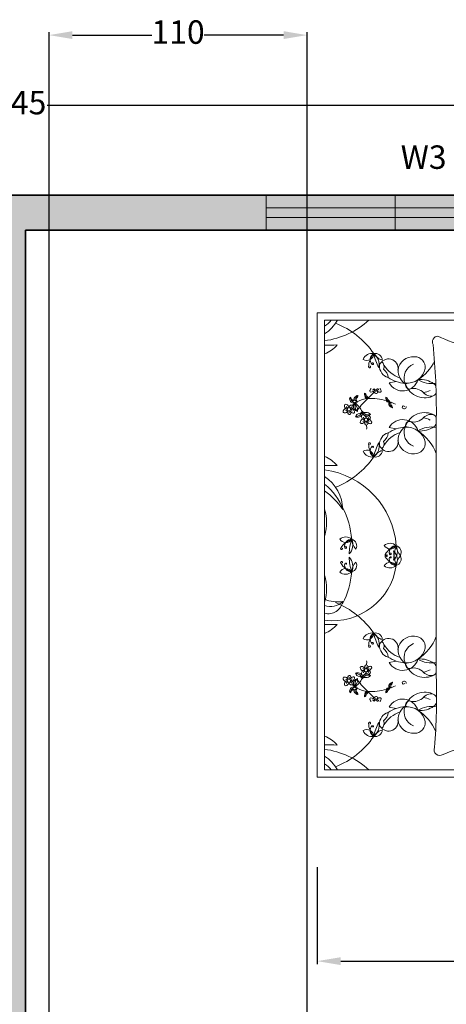
# Model space of a CAD drawing. Units: centimetres. Extents: x 2401 to 3632, y 2122 to 3526.
# Tile 9 of 10: x 2873 to 3055, y 3106 to 3526. Entities that reach past the tile are written whole.
import ezdxf

# ---------------------------------------------------------------- set-up
doc = ezdxf.new("R2010")
doc.units = ezdxf.units.CM
for name, color, linetype, lineweight in [('A-ANNO-DIMS', 9, 'Continuous', 18), ('A-ANNO-TEXT', 9, 'Continuous', 18), ('A-FURN', 9, 'Continuous', 18), ('A-GLAZ', 4, 'Continuous', 18), ('A-WALL', 7, 'Continuous', 35)]:
    doc.layers.add(name, color=color, linetype=linetype, lineweight=lineweight)
doc.layers.add('A-GLAZ-PATT', color=251, linetype='Continuous', lineweight=13, true_color=0x636466)
doc.layers.add('A-WALL-PATT', color=18, linetype='Continuous', lineweight=13, true_color=0x000000)
doc.styles.get("Standard").update_dxf_attribs({"font": 'arial.ttf'})
doc.dimstyles.new('ISO-25', dxfattribs={"dimtxt": 10, "dimasz": 10, "dimexe": 1.25, "dimexo": 0.625, "dimtad": 0, "dimtxsty": 'Standard', "dimcen": 2.5, "dimadec": 0, "dimazin": 0, "dimtfac": 1, "dimtmove": 0, "dimatfit": 3, "dimfxl": 1, "dimarcsym": 0})

# ---------------------------------------------------------------- blocks, each defined once
blk = doc.blocks.new('bed')
for p, q in [((3025.77, 3949.95), (3025.77, 3649.95)), ((3000.77, 3900.35), (3000.77, 3939.55)), ((2981.17, 3919.95), (3020.37, 3919.95)), ((2770.64, 3910.36), (2878.71, 3910.36)), ((2770.64, 3691.65), (2770.64, 3910.36)), ((2878.71, 3910.36), (2878.71, 3893.39)), ((2774.11, 3906.88), (2774.11, 3695.12)), ((2875.23, 3906.88), (2774.11, 3906.88)), ((2875.23, 3893.39), (2875.23, 3906.88)), ((2856.25, 3708.31), (2856.25, 3893.41)), ((2860, 3708.59), (2860, 3893.41)), ((2937.86, 3890.21), (2940.29, 3892.64)), ((2940.29, 3892.64), (2953.05, 3881.7)), ((2939.08, 3878.06), (2937.86, 3890.21)), ((3025.77, 3889.95), (2943.43, 3889.95)), ((2978.36, 3889.95), (2978.36, 3709.95)), ((3021.92, 3709.95), (3021.92, 3889.95)), ((2804.53, 3877.32), (2807.92, 3877.98)), ((2937.86, 3862.87), (2939.08, 3878.06)), ((2953.05, 3881.7), (2961.55, 3870.16)), ((2961.55, 3870.16), (2969.44, 3848.28)), ((2826.78, 3739.05), (2826.78, 3860.86)), ((2936.04, 3849.5), (2937.86, 3862.87)), ((2804.53, 3856.35), (2807.92, 3855.69)), ((2932.4, 3841.6), (2936.04, 3849.5)), ((2969.44, 3848.28), (2978.36, 3815.57)), ((2929.97, 3831.88), (2932.4, 3841.6)), ((2937.86, 3830.66), (2929.97, 3831.88)), ((2955.47, 3823.98), (2937.86, 3830.66)), ((2950.29, 3711.02), (2949.82, 3826.13)), ((2953.37, 3711.03), (2952.92, 3824.95)), ((2978.36, 3807.54), (2955.47, 3823.98)), ((2962.82, 3710.88), (2961.28, 3819.81)), ((2965.89, 3710.76), (2964.4, 3817.57)), ((2804.53, 3745.65), (2807.92, 3746.31)), ((2804.53, 3724.68), (2807.92, 3724.02)), ((2875.23, 3695.12), (2875.23, 3708.35)), ((2878.71, 3708.28), (2878.71, 3691.65)), ((3000.77, 3699.55), (3000.77, 3660.35)), ((2774.11, 3695.12), (2875.23, 3695.12)), ((2878.71, 3691.65), (2770.64, 3691.65)), ((2981.17, 3679.95), (3020.37, 3679.95))]:
    blk.add_line(p, q)
for points in [[(2975.77, 3889.95), (2975.77, 3949.95), (3025.77, 3949.95)], [(3000.77, 3919.95), (2994.7, 3916.45)], [(3000.77, 3919.95), (3006.83, 3916.45)], [(3025.77, 3709.95), (2975.77, 3709.95), (2975.77, 3649.95), (3025.77, 3649.95)], [(3000.77, 3679.95), (2994.7, 3683.45)], [(3000.77, 3679.95), (3006.83, 3683.45)]]:
    blk.add_lwpolyline(points)
for points in [[(2912.82, 3893.27, 0.001242), (2855.9, 3893.41, -0.127202), (2827.53, 3899.43)], [(3018.29, 3872.72, 0.074897), (2998.69, 3872.36, -0.472817)], [(2997.6, 3801.36, 0.14099), (3017.59, 3800.76, 0.235245)], [(2997.6, 3788.55, -0.14099), (3017.59, 3789.15, -0.235245)], [(3018.29, 3727.19, -0.074897), (2998.69, 3727.55, 0.472817)], [(2862.36, 3708.67, 0.056112), (2845.85, 3706.5, 0.095341), (2829.95, 3702.28)]]:
    blk.add_lwpolyline(points, format="xyb")
for centre, radius in [((3000.77, 3919.95), 14), ((3000.77, 3919.95), 7), ((2785.6, 3864.98), 0.764), ((2793.66, 3859.99), 0.764), ((2793.66, 3742.02), 0.764), ((2785.6, 3737.02), 0.764), ((3000.77, 3679.95), 14), ((3000.77, 3679.95), 7)]:
    blk.add_circle(centre, radius)
for centre, radius, start, end in [((2760.03, 3923.26), 23.79, 306.3036, 316.4814), ((2763.59, 3916.39), 19.09, 303.4617, 330.1116), ((2768.83, 3936.05), 39.18, 277.745, 311.8856), ((2764.96, 3869.02), 39.18, 34.3865, 68.5908), ((2827.73, 3896.66), 2.77, 93.98, 207.3412), ((2768, 3905.7), 15.93, 292.5547, 318.9546), ((2776.56, 3949.33), 54.2, 267.4081, 273.6519), ((2514.5, 3864.44), 312.3, 359.3433, 5.6887), ((2932.84, 4167.71), 275.17, 265.8294, 271.553), ((3046.53, 3887.51), 113.22, 177.4519, 191.3392), ((2796.37, 3886.9), 4.34, 77.7115, 159.0387), ((2794.02, 3891.25), 3.27, 238.4633, 358.2869), ((2804.75, 3884.63), 9.91, 138.8402, 177.9352), ((2798.78, 3888.31), 3.2, 117.6827, 223.7762), ((2798.06, 3887.99), 3.25, 2.9516, 103.728), ((2824.04, 3897.09), 27.41, 192.5173, 207.1824), ((2793.67, 3886.12), 6.19, 345.4653, 54.2343), ((2803, 3894.63), 6.69, 211.3827, 255.2969), ((2804.28, 3884.18), 4.5, 350.264, 160.8688), ((2799.41, 3885.11), 2.76, 333.9755, 53.2681), ((2815.84, 3882.53), 7.17, 84.9449, 172.8857), ((2816.56, 3884.61), 5.07, 354.4856, 91.0538), ((2805.66, 3897.83), 22.71, 303.6671, 333.2997), ((2795.33, 3884.97), 0.487, 177.9352, 11.4834), ((2795.58, 3885.02), 0.236, 11.4834, 127.9409), ((2796.77, 3886.39), 0.424, 223.7762, 159.7183), ((2805.64, 3885.26), 5.62, 175.969, 254.3045), ((2798.17, 3879.2), 5.99, 6.1662, 51.5825), ((2814.2, 3893.11), 14.16, 211.2614, 251.7045), ((2817.43, 3883.78), 8.71, 182.3591, 234.0401), ((2818.55, 3879.71), 6.96, 111.5819, 201.4221), ((2812.81, 3886.16), 9.02, 265.2933, 346.921), ((2813.05, 3893.24), 16.1, 236.2883, 266.5076), ((2810.99, 3881.04), 7.46, 209.9085, 343.1337), ((2824.57, 3889.51), 12.43, 238.8218, 279.1554), ((2819.17, 3867.4), 11.57, 55.785, 94.7304), ((2775.06, 3890.75), 28.48, 313.1541, 322.0459), ((2796.01, 3873.64), 0.586, 142.4737, 265.053), ((2796.78, 3873.76), 1.26, 127.7621, 169.0403), ((2796.11, 3874.82), 1.78, 265.053, 338.3618), ((2798.46, 3872.39), 2.32, 113.4276, 137.6104), ((2798.2, 3874.8), 0.764, 183.2768, 356.7232), ((2798.76, 3873.41), 1.25, 139.7889, 227.6792), ((2795.81, 3873.43), 2.5, 353.0852, 15.7171), ((2797.45, 3873.13), 1.58, 350.3487, 43.6538), ((2800.38, 3874.76), 1.84, 198.7263, 262.5032), ((2798.92, 3873.91), 0.73, 1.1081, 91.8675), ((2800.29, 3873.51), 0.59, 255.2356, 54.9248), ((2799.38, 3873.74), 1.27, 11.5637, 52.6358), ((2814.13, 3876.31), 1.86, 167.3041, 285.1471), ((2819.17, 3867.4), 11.57, 122.7011, 126.3445), ((2821.34, 3879.88), 9.56, 199.2822, 299.1751), ((2816.22, 3868.58), 6.15, 41.5653, 105.1471), ((2819.61, 3881.32), 8.62, 277.436, 299.9149), ((2823.47, 3874.11), 3.61, 30.0293, 52.325), ((2786.72, 3869.91), 0.853, 124.3538, 214.3923), ((2787.97, 3869.78), 1.99, 190.3057, 287.1958), ((2788.54, 3870.49), 2.31, 176.9701, 248.2913), ((2805.02, 3882.67), 22.32, 212.6784, 216.3746), ((2787.76, 3869.95), 0.883, 216.3746, 291.7548), ((2789.87, 3869.34), 1.99, 122.8155, 187.3992), ((2788.34, 3868.51), 0.666, 289.3605, 111.7548), ((2788.84, 3868.51), 0.666, 221.8703, 44.2646), ((2790.75, 3869.08), 2.31, 109.4799, 177.6828), ((2789.51, 3870.54), 0.853, 56.8636, 146.9021), ((2789.95, 3869.59), 0.883, 148.8844, 224.2646), ((2808.3, 3858.51), 22.32, 145.1882, 148.8844), ((2795.58, 3857.56), 12.46, 94.756, 119.2041), ((2822.1, 3839.62), 40.99, 132.2412, 142.1744), ((2801.41, 3872.25), 8.46, 178.3264, 187.1302), ((2792.27, 3871.07), 1.58, 11.3256, 64.4621), ((2797.62, 3873.34), 4.74, 190.2588, 210.656), ((2794.44, 3871.41), 1.44, 188.3432, 274.2869), ((2795.7, 3872.2), 2.51, 210.656, 242.6341), ((2797.6, 3874.36), 4.82, 218.2101, 226.3071), ((2794.04, 3870.31), 0.611, 325.7657, 67.4417), ((2796.2, 3845.18), 24.85, 73.5842, 93.8277), ((2798.36, 3872.98), 0.658, 227.6792, 350.3487), ((2811.5, 3870.46), 8.46, 178.3264, 187.1302), ((2802.37, 3869.29), 1.58, 11.3256, 64.4621), ((2807.71, 3871.55), 4.74, 190.2588, 210.656), ((2804.53, 3869.62), 1.44, 188.3432, 274.2869), ((2805.8, 3870.42), 2.51, 210.656, 242.6341), ((2807.7, 3872.58), 4.82, 218.2101, 226.3071), ((2804.13, 3868.53), 0.611, 325.7657, 67.4417), ((2824.18, 3875.64), 4.49, 221.5653, 293.8354), ((2823.47, 3874.11), 3.61, 314.4517, 333.558), ((3021.8, 3862.02), 40.2, 165.1039, 191.0369), ((2990.83, 3834.5), 38.67, 65.1316, 101.7583), ((5873.3, 3707.37), 2859.79, 176.68521, 177.14978), ((2783.42, 3863.83), 0.586, 142.4737, 265.053), ((2784.19, 3863.94), 1.26, 61.2196, 169.0403), ((2783.52, 3865.01), 1.78, 265.053, 338.3618), ((2785.02, 3866.54), 1.51, 157.4086, 261.4386), ((2784.17, 3866.59), 0.757, 58.0499, 135.6268), ((2785.87, 3862.58), 2.32, 113.4276, 137.6104), ((2784.96, 3866.11), 0.506, 172.906, 277.132), ((2783.3, 3865.19), 2.41, 14.7558, 58.0499), ((2786.17, 3863.6), 1.25, 139.7889, 227.6792), ((2786.67, 3865.83), 1.04, 36.1046, 181.4281), ((2783.22, 3863.62), 2.5, 353.0852, 15.7171), ((2784.86, 3863.32), 1.58, 350.3487, 43.6538), ((2787.79, 3864.95), 1.84, 198.7263, 262.5032), ((2786.06, 3866.65), 1.05, 270.0645, 331.1507), ((2786.96, 3866.4), 1.2, 221.8413, 265.7877), ((2786.33, 3864.09), 0.73, 1.1081, 91.8675), ((2786.95, 3865.94), 0.749, 263.7526, 41.7054), ((2786.79, 3863.93), 1.27, 11.5637, 86.365), ((2795.58, 3857.56), 12.46, 124.0033, 132.4917), ((2787.7, 3863.7), 0.59, 255.2356, 54.9248), ((2782.77, 3855.98), 13.31, 63.7819, 68.2913), ((2789.87, 3866.22), 2.12, 128.3208, 208.8162), ((2790.26, 3866.38), 2.53, 207.7043, 254.3516), ((2791.86, 3866.57), 3.48, 157.2305, 229.0635), ((2790.69, 3867.72), 2.05, 174.4544, 220.6188), ((2779.03, 3856.28), 14.94, 30.544, 49.818), ((2787.26, 3864.79), 2.46, 340.0041, 40.6188), ((2805.85, 3867.41), 1.44, 147.5332, 233.4768), ((2804.7, 3867.58), 0.611, 354.3784, 96.0543), ((2807.15, 3868.15), 2.51, 179.1859, 211.164), ((2796.2, 3845.18), 24.85, 63.0032, 69.8941), ((2809.06, 3869.3), 4.74, 211.164, 231.5612), ((2809.89, 3873.16), 8.46, 234.6898, 243.4936), ((2809.96, 3868.8), 4.82, 195.5129, 203.6099), ((2804.54, 3865.66), 1.58, 357.3579, 50.4944), ((2811.3, 3865.97), 0.578, 12.7051, 190.4384), ((2811.66, 3866.04), 0.94, 190.4384, 10.4136), ((2911.57, 3860.44), 24.42, 336.2616, 11.3392), ((2785.77, 3863.16), 0.658, 227.6792, 350.3487), ((2788.61, 3864.93), 3.48, 270.278, 342.111), ((2790.93, 3860.58), 2.46, 98.7227, 159.3375), ((2789.7, 3863.74), 2.53, 244.9899, 291.6373), ((2790.25, 3865.04), 2.05, 278.7227, 324.8872), ((2789.89, 3863.37), 2.12, 290.5253, 358.5375), ((2792.24, 3858.95), 1.26, 61.2196, 169.0403), ((2791.57, 3860.01), 1.78, 265.053, 338.3618), ((2793.07, 3861.54), 1.51, 157.4086, 261.4386), ((2792.22, 3861.59), 0.757, 58.0499, 135.6268), ((2794.02, 3863.97), 2.12, 182.8499, 266.1226), ((2793.19, 3865.47), 2.05, 231.7607, 277.9252), ((2794.79, 3865.83), 3.48, 214.5369, 286.3699), ((2793.92, 3857.58), 2.32, 113.4276, 137.6104), ((2793.01, 3861.12), 0.506, 172.906, 277.132), ((2791.35, 3860.19), 2.41, 14.7558, 58.0499), ((2779.03, 3856.28), 14.94, 23.0501, 23.8477), ((2794.22, 3858.6), 1.25, 139.7889, 227.6792), ((2793.81, 3861), 2.46, 37.3105, 97.9252), ((2794.72, 3860.83), 1.04, 36.1046, 181.4281), ((2791.27, 3858.62), 2.5, 353.0852, 15.7171), ((2794.09, 3864.38), 2.53, 265.0106, 311.658), ((2792.91, 3858.32), 1.58, 350.3487, 43.6538), ((2795.84, 3859.95), 1.84, 198.7263, 262.5032), ((2794.11, 3861.65), 1.05, 270.0645, 331.1507), ((2795.01, 3861.4), 1.2, 221.8413, 265.7877), ((2794.38, 3859.1), 0.73, 1.1081, 91.8675), ((2795, 3860.95), 0.749, 263.7526, 41.7054), ((2794.84, 3858.93), 1.27, 11.5637, 86.365), ((2810.99, 3852.63), 7.46, 16.8663, 150.0915), ((2821.34, 3853.79), 9.56, 60.8249, 160.7178), ((2816.22, 3865.09), 6.15, 254.8529, 318.4347), ((2819.61, 3852.35), 8.62, 60.0851, 82.564), ((2824.18, 3858.03), 4.49, 66.1646, 138.4347), ((2823.47, 3859.56), 3.61, 23.229, 45.5483), ((2791.47, 3858.83), 0.586, 142.4737, 265.053), ((2793.82, 3858.17), 0.658, 227.6792, 350.3487), ((2779.03, 3856.28), 14.94, 357.1071, 4.7585), ((2795.75, 3858.7), 0.59, 255.2356, 54.9248), ((2813.05, 3840.43), 16.1, 93.4924, 123.7117), ((2817.43, 3849.89), 8.71, 125.9599, 177.6409), ((2818.55, 3853.96), 6.96, 158.5779, 248.4181), ((2812.81, 3847.51), 9.02, 13.079, 94.7067), ((2814.13, 3857.35), 1.86, 74.8529, 192.6959), ((2819.17, 3866.26), 11.57, 233.6555, 237.2989), ((2824.57, 3844.16), 12.43, 79.7133, 121.1782), ((2819.17, 3866.26), 11.57, 265.2696, 304.215), ((2805.66, 3835.83), 22.71, 21.4941, 56.3329), ((2823.47, 3859.56), 3.61, 307.675, 336.7144), ((3050.38, 3840.86), 69.73, 168.0397, 199.2615), ((2805.64, 3848.41), 5.62, 105.6955, 184.031), ((2804.28, 3849.49), 4.5, 199.1312, 9.736), ((2798.17, 3854.46), 5.99, 308.4175, 353.8338), ((2814.2, 3840.56), 14.16, 108.2955, 148.7386), ((2815.84, 3851.14), 7.17, 187.1143, 275.0551), ((3043.34, 3811.05), 116.34, 160.1194, 169.3383), ((2794.02, 3842.42), 3.27, 1.7131, 121.5367), ((2795.33, 3848.7), 0.487, 348.5166, 182.0648), ((2804.75, 3849.04), 9.91, 182.0648, 221.1598), ((2795.58, 3848.65), 0.236, 232.0591, 348.5166), ((2798.78, 3845.36), 3.2, 136.2238, 242.3173), ((2796.93, 3847.24), 0.255, 200.2667, 136.2271), ((2793.67, 3847.55), 6.19, 305.7657, 14.5347), ((2824.04, 3836.58), 27.41, 152.8176, 167.4827), ((2798.06, 3845.68), 3.25, 256.272, 357.0484), ((2803, 3839.04), 6.69, 104.7031, 148.6173), ((2799.41, 3848.56), 2.76, 306.7319, 26.0245), ((2816.56, 3849.06), 5.07, 268.9462, 5.5144), ((2909.73, 3831.62), 108.8, 352.2196, 9.497), ((2768, 3827.97), 15.93, 41.0454, 67.4453), ((2764.96, 3864.65), 39.18, 291.4092, 325.6135), ((2796.37, 3846.77), 4.34, 200.9613, 282.2885), ((2776.56, 3784.33), 54.2, 86.3481, 92.5919), ((2768.83, 3797.62), 39.18, 4.4623, 82.255), ((2763.59, 3817.28), 19.09, 1.272, 56.5383), ((2929.73, 3832.56), 0.724, 178.8623, 289.7536), ((2760.03, 3810.41), 23.79, 17.8504, 53.6964), ((2753.34, 3797.91), 35.39, 34.0123, 54.053), ((2753.52, 3811.58), 21.54, 343.5431, 17.0202), ((2747.85, 3800.62), 39.18, 4.4623, 27.4146), ((3035.15, 3812.63), 52.9, 169.8617, 193.6238), ((2964.72, 3808.64), 53.46, 351.5249, 13.96), ((2742.41, 3803.04), 31.85, 4.3787, 5.6357), ((2720.59, 3786.27), 56.92, 19.7217, 19.9028), ((2783.99, 3800.45), 4.34, 47.7873, 129.1145), ((2784.12, 3805.39), 3.27, 208.5391, 328.3627), ((2790.12, 3794.3), 9.91, 108.9159, 148.011), ((2786.78, 3800.47), 3.2, 87.7585, 193.852), ((2813.06, 3795.47), 27.41, 162.593, 177.2582), ((2781.26, 3801.12), 6.19, 315.5411, 24.3101), ((2793.6, 3803.84), 6.69, 181.4585, 225.3727), ((2786, 3800.55), 3.25, 333.0274, 73.8037), ((2782.13, 3799.29), 0.487, 148.011, 341.5592), ((2782.37, 3799.21), 0.236, 341.5592, 98.0167), ((2784.08, 3799.8), 0.424, 193.852, 129.9245), ((2804.97, 3797.45), 4.34, 47.7873, 129.1145), ((2805.11, 3802.39), 3.27, 208.5391, 328.3627), ((2811.1, 3791.3), 9.91, 108.9159, 148.011), ((2807.77, 3797.47), 3.2, 87.7585, 193.852), ((2802.25, 3798.12), 6.19, 315.5411, 24.3101), ((2834.04, 3792.47), 27.41, 162.593, 177.2582), ((2806.98, 3797.55), 3.25, 333.0274, 73.8037), ((2814.58, 3800.84), 6.69, 181.4585, 225.3727), ((2987.57, 3836.72), 36.76, 264.0129, 285.8293), ((2813.06, 3796.53), 27.41, 182.7418, 197.407), ((2781.26, 3790.88), 6.19, 335.6899, 44.4589), ((2803.11, 3796.29), 0.487, 148.011, 341.5592), ((2803.11, 3795.71), 0.487, 18.4408, 211.989), ((2811.1, 3800.7), 9.91, 211.989, 251.0841), ((2803.35, 3796.21), 0.236, 341.5592, 98.0167), ((2803.35, 3795.79), 0.236, 261.9833, 18.4408), ((2807.77, 3794.53), 3.2, 166.148, 272.2415), ((2805.07, 3796.8), 0.424, 193.852, 129.9245), ((2805.23, 3795.24), 0.255, 230.1909, 166.0209), ((2802.25, 3793.88), 6.19, 335.6899, 44.4589), ((2834.04, 3799.53), 27.41, 182.7418, 197.407), ((2806.98, 3794.45), 3.25, 286.1963, 26.9726), ((2814.58, 3791.16), 6.69, 134.6273, 178.5415), ((2777.88, 3795.65), 30.32, 262.8636, 351.8197), ((2784.12, 3786.62), 3.27, 31.6373, 151.4609), ((2782.13, 3792.71), 0.487, 18.4408, 211.989), ((2790.12, 3797.71), 9.91, 211.989, 251.0841), ((2782.37, 3792.79), 0.236, 261.9833, 18.4408), ((2786.78, 3791.54), 3.2, 166.148, 272.2415), ((2784.25, 3792.24), 0.255, 230.1909, 166.0209), ((2793.6, 3788.16), 6.69, 134.6273, 178.5415), ((2786, 3791.45), 3.25, 286.1963, 26.9726), ((2805.11, 3789.62), 3.27, 31.6373, 151.4609), ((2804.97, 3794.55), 4.34, 230.8855, 312.2127), ((2998.15, 3783.03), 15.9, 155.0183, 198.5407), ((2987.57, 3753.18), 36.76, 74.1707, 95.9871), ((2753.52, 3780.42), 21.54, 342.9798, 16.4569), ((2742.41, 3788.96), 31.85, 354.3643, 355.6213), ((2720.59, 3805.74), 56.92, 340.0972, 340.2783), ((2783.99, 3791.55), 4.34, 230.8855, 312.2127), ((2747.85, 3791.38), 39.18, 332.5854, 355.5377), ((3003.33, 3785.03), 14.84, 333.3437, 16.1026), ((2780.65, 3791.73), 17.54, 248.117, 276.6195), ((2775.77, 3775.64), 7.03, 256.3898, 349.0739), ((2776.73, 3780.92), 8.89, 252.8609, 311.9049), ((2764.96, 3737.36), 39.18, 34.3865, 68.5908), ((3018.84, 3755.24), 38.19, 153.8761, 196.1746), ((2965.8, 3762.79), 52.74, 346.3427, 11.1841), ((2776.56, 3817.67), 54.2, 267.4081, 273.6519), ((2768, 3774.04), 15.93, 292.5547, 318.9546), ((2796.37, 3755.24), 4.34, 77.7115, 159.0387), ((2794.02, 3759.58), 3.27, 238.4633, 358.2869), ((2804.75, 3752.96), 9.91, 138.8402, 177.9352), ((2798.78, 3756.64), 3.2, 117.6827, 223.7762), ((2798.06, 3756.33), 3.25, 2.9516, 103.728), ((2803, 3762.97), 6.69, 211.3827, 255.2969), ((2793.67, 3754.46), 6.19, 345.4653, 54.2343), ((2824.04, 3765.42), 27.41, 192.5173, 207.1824), ((2815.84, 3750.86), 7.17, 84.9449, 172.8857), ((2816.56, 3752.94), 5.07, 354.4856, 91.0538), ((2805.66, 3766.17), 22.71, 303.6671, 338.5059), ((2795.33, 3753.3), 0.487, 177.9352, 11.4834), ((2795.58, 3753.35), 0.236, 11.4834, 127.9409), ((2796.77, 3754.72), 0.424, 223.7762, 159.7183), ((2805.64, 3753.59), 5.62, 175.969, 254.3045), ((2804.28, 3752.51), 4.5, 350.264, 160.8688), ((2799.41, 3753.44), 2.76, 333.9755, 53.2681), ((2814.2, 3761.44), 14.16, 211.2614, 251.7045), ((2818.55, 3748.05), 6.96, 111.5819, 201.4221), ((2798.17, 3747.54), 5.99, 6.1662, 51.5825), ((2813.05, 3761.57), 16.1, 236.2883, 266.5076), ((2817.43, 3752.11), 8.71, 182.3591, 234.0401), ((2812.81, 3754.5), 9.02, 265.2933, 346.921), ((5873.3, 3892.54), 2859.79, 182.85022, 183.31479), ((2791.47, 3743.17), 0.586, 94.947, 217.5263), ((2791.57, 3741.99), 1.78, 21.6382, 94.947), ((2794.22, 3743.4), 1.25, 132.3208, 220.2111), ((2793.82, 3743.84), 0.658, 9.6513, 132.3208), ((2791.27, 3743.38), 2.5, 344.2829, 6.9148), ((2779.03, 3745.73), 14.94, 355.2415, 2.8929), ((2792.91, 3743.68), 1.58, 316.3462, 9.6513), ((2795.84, 3742.05), 1.84, 97.4968, 161.2737), ((2795.75, 3743.3), 0.59, 305.0752, 104.7644), ((2810.99, 3749.37), 7.46, 209.9085, 343.1337), ((2814.13, 3744.65), 1.86, 167.3041, 285.1471), ((2819.17, 3735.74), 11.57, 122.7011, 126.3445), ((2821.34, 3748.21), 9.56, 199.2822, 299.1751), ((2824.57, 3757.84), 12.43, 238.8218, 280.2867), ((2819.17, 3735.74), 11.57, 55.785, 94.7304), ((2823.47, 3742.45), 3.61, 23.2856, 52.325), ((3021.8, 3737.89), 40.2, 168.9631, 194.8961), ((2783.42, 3738.18), 0.586, 94.947, 217.5263), ((2783.52, 3736.99), 1.78, 21.6382, 94.947), ((2786.17, 3738.4), 1.25, 132.3208, 220.2111), ((2785.77, 3738.84), 0.658, 9.6513, 132.3208), ((2783.22, 3738.38), 2.5, 344.2829, 6.9148), ((2784.86, 3738.68), 1.58, 316.3462, 9.6513), ((2787.79, 3737.05), 1.84, 97.4968, 161.2737), ((2787.7, 3738.3), 0.59, 305.0752, 104.7644), ((2789.7, 3738.26), 2.53, 68.3627, 115.0101), ((2788.61, 3737.07), 3.48, 17.889, 89.722), ((2790.93, 3741.42), 2.46, 200.6625, 261.2773), ((2790.25, 3736.96), 2.05, 35.1128, 81.2773), ((2789.89, 3738.63), 2.12, 1.4625, 69.4747), ((2792.24, 3743.06), 1.26, 190.9597, 298.7804), ((2793.07, 3740.46), 1.51, 98.5614, 202.5914), ((2792.22, 3740.41), 0.757, 224.3732, 301.9501), ((2794.02, 3738.03), 2.12, 93.8774, 177.1501), ((2794.79, 3736.17), 3.48, 73.6301, 145.4631), ((2793.92, 3744.42), 2.32, 222.3896, 246.5724), ((2793.01, 3740.89), 0.506, 82.868, 187.094), ((2791.35, 3741.81), 2.41, 301.9501, 345.2442), ((2779.03, 3745.73), 14.94, 336.1523, 336.9499), ((2793.81, 3741), 2.46, 262.0748, 322.6895), ((2794.72, 3741.17), 1.04, 178.5719, 323.8954), ((2794.09, 3737.62), 2.53, 48.342, 94.9894), ((2795.01, 3740.6), 1.2, 94.2123, 138.1587), ((2794.11, 3740.35), 1.05, 28.8493, 89.9355), ((2794.38, 3742.91), 0.73, 268.1325, 358.8919), ((2794.84, 3743.07), 1.27, 273.635, 348.4363), ((2795, 3741.06), 0.749, 318.2946, 96.2474), ((2816.22, 3736.91), 6.15, 41.5653, 105.1471), ((2819.61, 3749.66), 8.62, 277.436, 299.9149), ((2824.18, 3743.97), 4.49, 221.5653, 293.8354), ((2535.01, 3729.86), 291.92, 355.2402, 1.8035), ((2823.47, 3742.45), 3.61, 314.4517, 336.7144), ((2784.19, 3738.06), 1.26, 190.9597, 298.7804), ((2785.02, 3735.46), 1.51, 98.5614, 202.5914), ((2784.17, 3735.41), 0.757, 224.3732, 301.9501), ((2785.87, 3739.42), 2.32, 222.3896, 246.5724), ((2784.96, 3735.89), 0.506, 82.868, 187.094), ((2783.3, 3736.82), 2.41, 301.9501, 345.2442), ((2786.67, 3736.18), 1.04, 178.5719, 323.8954), ((2787.97, 3732.22), 1.99, 72.8042, 169.6943), ((2786.96, 3735.61), 1.2, 94.2123, 138.1587), ((2786.06, 3735.36), 1.05, 28.8493, 89.9355), ((2786.33, 3737.91), 0.73, 268.1325, 358.8919), ((2786.79, 3738.08), 1.27, 273.635, 348.4363), ((2786.95, 3736.06), 0.749, 318.2946, 96.2474), ((2795.58, 3744.44), 12.46, 227.5083, 235.9967), ((2782.77, 3746.02), 13.31, 291.7087, 296.2181), ((2789.87, 3735.78), 2.12, 151.1838, 231.6792), ((2790.26, 3735.62), 2.53, 105.6484, 152.2957), ((2788.34, 3733.49), 0.666, 248.2452, 70.6395), ((2788.84, 3733.49), 0.666, 315.7354, 138.1297), ((2791.86, 3735.43), 3.48, 130.9365, 202.7695), ((2790.69, 3734.28), 2.05, 139.3812, 185.5456), ((2779.03, 3745.73), 14.94, 310.182, 329.456), ((2787.26, 3737.22), 2.46, 319.3812, 19.9959), ((2822.1, 3762.38), 40.99, 217.8256, 227.7588), ((2793.19, 3736.53), 2.05, 82.0748, 128.2393), ((2805.85, 3734.59), 1.44, 126.5232, 212.4668), ((2807.15, 3733.85), 2.51, 148.836, 180.8141), ((2804.7, 3734.43), 0.611, 263.9457, 5.6216), ((2796.2, 3756.82), 24.85, 290.1059, 296.9968), ((2809.06, 3732.7), 4.74, 128.4388, 148.836), ((2809.89, 3728.84), 8.46, 116.5064, 125.3102), ((2809.96, 3733.2), 4.82, 156.3901, 164.4871), ((2804.54, 3736.34), 1.58, 309.5056, 2.6421), ((2811.3, 3736.03), 0.578, 169.5616, 347.2949), ((2811.66, 3735.96), 0.94, 349.5864, 169.5616), ((2786.72, 3732.09), 0.853, 145.6077, 235.6462), ((2788.54, 3731.51), 2.31, 111.7087, 183.0299), ((2805.02, 3719.34), 22.32, 143.6254, 147.3216), ((2787.76, 3732.05), 0.883, 68.2452, 143.6254), ((2789.87, 3732.67), 1.99, 172.6008, 237.1845), ((2790.75, 3732.92), 2.31, 182.3172, 250.5201), ((2789.51, 3731.46), 0.853, 213.0979, 303.1364), ((2789.95, 3732.41), 0.883, 135.7354, 211.1156), ((2808.3, 3743.49), 22.32, 211.1156, 214.8118), ((2795.58, 3744.44), 12.46, 240.7959, 265.244), ((2797.62, 3728.66), 4.74, 149.344, 169.7412), ((2801.41, 3729.75), 8.46, 172.8698, 181.6736), ((2792.27, 3730.93), 1.58, 295.5379, 348.6744), ((2794.44, 3730.6), 1.44, 85.7131, 171.6568), ((2795.7, 3729.8), 2.51, 117.3659, 149.344), ((2797.6, 3727.64), 4.82, 133.6929, 141.7899), ((2794.04, 3731.69), 0.611, 292.5583, 34.2343), ((2796.2, 3756.82), 24.85, 266.1723, 286.4158), ((2775.06, 3711.25), 28.48, 37.9541, 46.8459), ((2798.76, 3728.59), 1.25, 132.3208, 220.2111), ((2798.36, 3729.03), 0.658, 9.6513, 132.3208), ((2811.5, 3731.54), 8.46, 172.8698, 181.6736), ((2807.71, 3730.45), 4.74, 149.344, 169.7412), ((2802.37, 3732.72), 1.58, 295.5379, 348.6744), ((2804.53, 3732.38), 1.44, 85.7131, 171.6568), ((2805.8, 3731.59), 2.51, 117.3659, 149.344), ((2807.7, 3729.43), 4.82, 133.6929, 141.7899), ((2804.13, 3733.47), 0.611, 292.5583, 34.2343), ((2821.34, 3722.12), 9.56, 60.8249, 160.7178), ((2824.18, 3726.36), 4.49, 66.1646, 138.4347), ((2823.47, 3727.89), 3.61, 16.6343, 45.5483), ((2990.83, 3765.41), 38.67, 258.2417, 294.8684), ((2796.01, 3728.36), 0.586, 94.947, 217.5263), ((2796.78, 3728.25), 1.26, 190.9597, 232.2379), ((2796.11, 3727.18), 1.78, 21.6382, 94.947), ((2798.46, 3729.61), 2.32, 222.3896, 246.5724), ((2798.2, 3727.21), 0.764, 3.2768, 176.7232), ((2795.81, 3728.57), 2.5, 344.2829, 6.9148), ((2797.45, 3728.87), 1.58, 316.3462, 9.6513), ((2800.38, 3727.24), 1.84, 97.4968, 161.2737), ((2798.92, 3728.1), 0.73, 268.1325, 358.8919), ((2800.29, 3728.49), 0.59, 305.0752, 104.7644), ((2799.38, 3728.26), 1.27, 307.3642, 348.4363), ((2813.05, 3708.76), 16.1, 93.4924, 123.7117), ((2810.99, 3720.97), 7.46, 16.8663, 150.0915), ((2817.43, 3718.23), 8.71, 125.9599, 177.6409), ((2818.55, 3722.29), 6.96, 158.5779, 248.4181), ((2812.81, 3715.84), 9.02, 13.079, 94.7067), ((2814.13, 3725.69), 1.86, 74.8529, 192.6959), ((2819.17, 3734.6), 11.57, 233.6555, 237.2989), ((2816.22, 3733.42), 6.15, 254.8529, 318.4347), ((2824.57, 3712.5), 12.43, 79.249, 121.1782), ((2819.17, 3734.6), 11.57, 265.2696, 304.215), ((2819.61, 3720.68), 8.62, 60.0851, 82.564), ((2823.47, 3727.89), 3.61, 307.675, 342.5814), ((2805.64, 3716.74), 5.62, 105.6955, 184.031), ((2798.17, 3722.8), 5.99, 308.4175, 353.8338), ((2814.2, 3708.9), 14.16, 108.2955, 148.7386), ((2805.66, 3704.17), 22.71, 23.6453, 56.3329), ((2795.33, 3717.04), 0.487, 348.5166, 182.0648), ((2804.75, 3717.37), 9.91, 182.0648, 221.1598), ((2795.58, 3716.99), 0.236, 232.0591, 348.5166), ((2798.78, 3713.69), 3.2, 136.2238, 242.3173), ((2796.93, 3715.57), 0.255, 200.2667, 136.2271), ((2824.04, 3704.91), 27.41, 152.8176, 167.4827), ((2793.67, 3715.88), 6.19, 305.7657, 14.5347), ((2804.28, 3717.82), 4.5, 199.1312, 9.736), ((2799.41, 3716.9), 2.76, 306.7319, 26.0245), ((2815.84, 3719.47), 7.17, 187.1143, 275.0551), ((2816.56, 3717.4), 5.07, 268.9462, 5.5144), ((2768, 3696.3), 15.93, 41.0454, 67.4453), ((2764.96, 3732.98), 39.18, 291.4092, 325.6135), ((2794.02, 3710.76), 3.27, 1.7131, 121.5367), ((2796.37, 3715.1), 4.34, 200.9613, 282.2885), ((2803, 3707.37), 6.69, 104.7031, 148.6173), ((2798.06, 3714.01), 3.25, 256.272, 357.0484), ((2922.1, 3008.05), 703.17, 89.11454, 94.87351), ((2941.69, 3172.15), 539.05, 86.1, 90.9282), ((2776.56, 3652.67), 54.2, 86.3481, 92.5919), ((2768.83, 3665.96), 39.18, 48.1144, 82.255), ((2828.43, 3704.55), 2.73, 156.5219, 303.8264), ((2763.59, 3685.61), 19.09, 29.8884, 56.5383), ((2760.03, 3678.74), 23.79, 43.5186, 53.6964)]:
    blk.add_arc(centre, radius, start, end)
blk = doc.blocks.new('*D17')
at = {"layer": 'A-ANNO-DIMS', "color": 0, "lineweight": -2, "transparency": 16777216}
for p, q in [((2500.44, 3451.73), (2500.44, 3490.46)), ((3245.44, 3451.73), (3245.44, 3490.46)), ((2510.44, 3489.21), (2861.27, 3489.21)), ((3235.44, 3489.21), (2884.6, 3489.21))]:
    blk.add_line(p, q, dxfattribs=at)
at = {"layer": 'A-ANNO-DIMS', "color": 0, "transparency": 16777216}
for points in [[(2510.44, 3490.88), (2510.44, 3487.55), (2500.44, 3489.21)], [(3235.44, 3490.88), (3235.44, 3487.55), (3245.44, 3489.21)]]:
    blk.add_solid(points, dxfattribs=at)
at = {"layer": 'Defpoints', "color": 0, "transparency": 16777216}
for p in [(3245.44, 3489.21), (2500.44, 3451.1), (3245.44, 3451.1)]:
    blk.add_point(p, dxfattribs=at)
at = {"layer": 'A-ANNO-DIMS', "color": 0, "transparency": 16777216, "insert": (2872.94, 3489.21), "char_height": 10, "attachment_point": 5}
blk.add_mtext('745', dxfattribs=at)
blk = doc.blocks.new('WIN-1500-3P')
for p, q in [((0, 15), (0, 0)), ((55, 15), (55, 0)), ((95, 15), (95, 0)), ((150, 15), (150, 0)), ((0, 9.5), (150, 9.5)), ((0, 5.5), (150, 5.5))]:
    blk.add_line(p, q)
blk = doc.blocks.new('*D25')
at = {"layer": 'A-ANNO-DIMS', "color": 0, "lineweight": -2, "transparency": 16777216}
for p, q in [((2999.75, 3164.85), (2999.75, 3123.53)), ((3230.44, 3164.85), (3230.44, 3123.53)), ((3009.75, 3124.78), (3086.16, 3124.78)), ((3220.44, 3124.78), (3144.02, 3124.78))]:
    blk.add_line(p, q, dxfattribs=at)
at = {"layer": 'A-ANNO-DIMS', "color": 0, "transparency": 16777216}
for points in [[(3009.75, 3126.45), (3009.75, 3123.12), (2999.75, 3124.78)], [(3220.44, 3126.45), (3220.44, 3123.12), (3230.44, 3124.78)]]:
    blk.add_solid(points, dxfattribs=at)
at = {"layer": 'Defpoints', "color": 0, "transparency": 16777216}
for p in [(2999.75, 3165.47), (3230.44, 3165.47), (3230.44, 3124.78)]:
    blk.add_point(p, dxfattribs=at)
at = {"layer": 'A-ANNO-DIMS', "color": 0, "transparency": 16777216, "insert": (3115.09, 3124.78), "char_height": 10, "attachment_point": 5}
blk.add_mtext('231 TYP.', dxfattribs=at)
blk = doc.blocks.new('*D52')
at = {"layer": 'A-ANNO-DIMS', "color": 0, "lineweight": -2, "transparency": 16777216}
for p, q in [((2885.44, 2411.73), (2885.44, 3520.5)), ((2895.44, 3519.25), (2929.25, 3519.25)), ((2985.44, 3519.25), (2951.62, 3519.25)), ((2995.44, 2591.73), (2995.44, 3520.5))]:
    blk.add_line(p, q, dxfattribs=at)
at = {"layer": 'A-ANNO-DIMS', "color": 0, "transparency": 16777216}
for points in [[(2895.44, 3520.92), (2895.44, 3517.59), (2885.44, 3519.25)], [(2985.44, 3520.92), (2985.44, 3517.59), (2995.44, 3519.25)]]:
    blk.add_solid(points, dxfattribs=at)
at = {"layer": 'Defpoints', "color": 0, "transparency": 16777216}
for p in [(2995.44, 3519.25), (2995.44, 2591.1), (2885.44, 2411.1)]:
    blk.add_point(p, dxfattribs=at)
at = {"layer": 'A-ANNO-DIMS', "color": 0, "transparency": 16777216, "insert": (2940.44, 3519.25), "char_height": 10, "attachment_point": 5}
blk.add_mtext('110', dxfattribs=at)

msp = doc.modelspace()

# ---------------------------------------------------------------- hatches: boundary and pattern name
at = {"layer": 'A-GLAZ-PATT'}
h = msp.add_hatch(color=256, dxfattribs=at)
h.dxf.hatch_style = 1
h.paths.add_polyline_path([(2505.936, 3356.104), (2500.436, 3356.104), (2500.436, 3301.104), (2505.936, 3301.104)])
h.paths.add_polyline_path([(2509.936, 3356.104), (2505.936, 3356.104), (2505.936, 3301.104), (2509.936, 3301.104)])
h.paths.add_polyline_path([(2515.436, 3335.674), (2515.436, 3356.104), (2509.936, 3356.104), (2509.936, 3301.104), (2515.436, 3301.104)])
h.paths.add_polyline_path([(2509.936, 3301.104), (2505.936, 3301.104), (2505.936, 3261.104), (2509.936, 3261.104)])
h.paths.add_polyline_path([(2515.436, 3301.104), (2509.936, 3301.104), (2509.936, 3261.104), (2515.436, 3261.104)])
h.paths.add_polyline_path([(2505.936, 3301.104), (2500.436, 3301.104), (2500.436, 3261.104), (2505.936, 3261.104)])
h.paths.add_polyline_path([(2515.436, 3261.104), (2509.936, 3261.104), (2509.936, 3206.104), (2515.436, 3206.104)])
h.paths.add_polyline_path([(2505.936, 3261.104), (2500.436, 3261.104), (2500.436, 3206.104), (2505.936, 3206.104)])
h.paths.add_polyline_path([(2509.936, 3261.104), (2505.936, 3261.104), (2505.936, 3206.104), (2509.936, 3206.104)])
h.paths.add_polyline_path([(3127.936, 3451.104), (3072.936, 3451.104), (3072.936, 3445.604), (3127.936, 3445.604)])
h.paths.add_polyline_path([(3032.936, 3441.604), (2977.936, 3441.604), (2977.936, 3436.104), (3032.936, 3436.104)])
h.paths.add_polyline_path([(3032.936, 3451.104), (2977.936, 3451.104), (2977.936, 3445.604), (3032.936, 3445.604)])
h.paths.add_polyline_path([(3032.936, 3445.604), (2977.936, 3445.604), (2977.936, 3441.604), (3032.936, 3441.604)])
h.paths.add_polyline_path([(3072.936, 3451.104), (3032.936, 3451.104), (3032.936, 3445.604), (3072.936, 3445.604)])
h.paths.add_polyline_path([(3072.936, 3445.604), (3032.936, 3445.604), (3032.936, 3441.604), (3072.936, 3441.604)])
h.paths.add_polyline_path([(3072.936, 3441.604), (3032.936, 3441.604), (3032.936, 3436.104), (3072.936, 3436.104)])
h.paths.add_polyline_path([(3127.936, 3441.604), (3072.936, 3441.604), (3072.936, 3436.104), (3127.936, 3436.104)])
h.paths.add_polyline_path([(3127.936, 3445.604), (3072.936, 3445.604), (3072.936, 3441.604), (3127.936, 3441.604)])
h.paths.add_polyline_path([(3245.436, 3356.104), (3239.936, 3356.104), (3239.936, 3301.104), (3245.436, 3301.104)])
h.paths.add_polyline_path([(3239.936, 3356.104), (3235.936, 3356.104), (3235.936, 3301.104), (3239.936, 3301.104)])
h.paths.add_polyline_path([(3235.936, 3356.104), (3230.436, 3356.104), (3230.436, 3301.104), (3235.936, 3301.104)])
h.paths.add_polyline_path([(3235.936, 3301.104), (3230.436, 3301.104), (3230.436, 3261.104), (3235.936, 3261.104)])
h.paths.add_polyline_path([(3239.936, 3301.104), (3235.936, 3301.104), (3235.936, 3261.104), (3239.936, 3261.104)])
h.paths.add_polyline_path([(3245.436, 3301.104), (3239.936, 3301.104), (3239.936, 3261.104), (3245.436, 3261.104)])
h.paths.add_polyline_path([(3245.436, 3261.104), (3239.936, 3261.104), (3239.936, 3206.104), (3245.436, 3206.104)])
h.paths.add_polyline_path([(3239.936, 3261.104), (3235.936, 3261.104), (3235.936, 3206.104), (3239.936, 3206.104)])
h.paths.add_polyline_path([(3235.936, 3261.104), (3230.436, 3261.104), (3230.436, 3206.104), (3235.936, 3206.104)])
h.paths.add_polyline_path([(3239.936, 3036.104), (3235.936, 3036.104), (3235.936, 2976.104), (3239.936, 2976.104)])
h.paths.add_polyline_path([(3235.936, 3036.104), (3230.436, 3036.104), (3230.436, 2976.104), (3235.936, 2976.104)])
h.paths.add_polyline_path([(3245.436, 3036.104), (3239.936, 3036.104), (3239.936, 2976.104), (3245.436, 2976.104)])
h.paths.add_polyline_path([(3235.936, 2836.104), (3230.436, 2836.104), (3230.436, 2781.104), (3235.936, 2781.104)])
h.paths.add_polyline_path([(3245.436, 2836.104), (3239.936, 2836.104), (3239.936, 2781.104), (3245.436, 2781.104)])
h.paths.add_polyline_path([(3239.936, 2836.104), (3235.936, 2836.104), (3235.936, 2781.104), (3239.936, 2781.104)])
h.paths.add_polyline_path([(3245.436, 2781.104), (3239.936, 2781.104), (3239.936, 2741.104), (3245.436, 2741.104)])
h.paths.add_polyline_path([(3239.936, 2781.104), (3235.936, 2781.104), (3235.936, 2741.104), (3239.936, 2741.104)])
h.paths.add_polyline_path([(3235.936, 2781.104), (3230.436, 2781.104), (3230.436, 2741.104), (3235.936, 2741.104)])
h.paths.add_polyline_path([(3245.436, 2741.104), (3239.936, 2741.104), (3239.936, 2686.104), (3245.436, 2686.104)])
h.paths.add_polyline_path([(3239.936, 2741.104), (3235.936, 2741.104), (3235.936, 2686.104), (3239.936, 2686.104)])
h.paths.add_polyline_path([(3235.936, 2741.104), (3230.436, 2741.104), (3230.436, 2686.104), (3235.936, 2686.104)])
h.paths.add_polyline_path([(3187.936, 2606.104), (3132.936, 2606.104), (3132.936, 2600.604), (3187.936, 2600.604)])
h.paths.add_polyline_path([(3187.936, 2600.604), (3132.936, 2600.604), (3132.936, 2596.604), (3187.936, 2596.604)])
h.paths.add_polyline_path([(3187.936, 2596.604), (3132.936, 2596.604), (3132.936, 2591.104), (3187.936, 2591.104)])
h.paths.add_polyline_path([(3132.936, 2596.604), (3092.936, 2596.604), (3092.936, 2591.104), (3132.936, 2591.104)])
h.paths.add_polyline_path([(3132.936, 2600.604), (3092.936, 2600.604), (3092.936, 2596.604), (3132.936, 2596.604)])
h.paths.add_polyline_path([(3132.936, 2606.104), (3092.936, 2606.104), (3092.936, 2600.604), (3132.936, 2600.604)])
h.paths.add_polyline_path([(3092.936, 2596.604), (3037.936, 2596.604), (3037.936, 2591.104), (3092.936, 2591.104)])
h.paths.add_polyline_path([(3092.936, 2600.604), (3037.936, 2600.604), (3037.936, 2596.604), (3092.936, 2596.604)])
h.paths.add_polyline_path([(3092.936, 2606.104), (3037.936, 2606.104), (3037.936, 2600.604), (3092.936, 2600.604)])
h.paths.add_polyline_path([(2803.613, 3432.66), (2826.471, 3432.66), (2826.471, 3453.267), (2803.613, 3453.267)], flags=9)
h.paths.add_polyline_path([(2904.038, 3087.418), (2926.896, 3087.418), (2926.896, 3108.025), (2904.038, 3108.025)], flags=9)
h.paths.add_polyline_path([(2801.908, 3105.391), (2824.766, 3105.391), (2824.766, 3125.998), (2801.908, 3125.998)], flags=9)
h.paths.add_polyline_path([(2757.576, 2660.284), (2780.434, 2660.284), (2780.434, 2680.892), (2757.576, 2680.892)], flags=9)
h.paths.add_polyline_path([(3004.446, 3080.825), (3027.304, 3080.825), (3027.304, 3101.432), (3004.446, 3101.432)], flags=9)
h.paths.add_polyline_path([(2805.63, 2777.019), (2828.489, 2777.019), (2828.489, 2797.626), (2805.63, 2797.626)], flags=9)
h.paths.add_polyline_path([(3094.334, 2572.754), (3128.823, 2572.754), (3128.823, 2593.361), (3094.334, 2593.361)], flags=9)
h.paths.add_polyline_path([(2931.792, 2588.154), (2946.88, 2588.154), (2946.88, 2608.761), (2931.792, 2608.761)], flags=9)
h.paths.add_polyline_path([(2582.951, 2415.87), (2664.015, 2415.87), (2664.015, 2453.184), (2582.951, 2453.184)], flags=9)
h.paths.add_polyline_path([(2622.234, 2685.113), (2683.168, 2685.113), (2683.168, 2722.427), (2622.234, 2722.427)], flags=9)
h.paths.add_polyline_path([(3027.646, 2511.408), (3088.58, 2511.408), (3088.58, 2548.722), (3027.646, 2548.722)], flags=9)
h.paths.add_polyline_path([(3020.004, 2720.966), (3092.521, 2720.966), (3092.521, 2758.281), (3020.004, 2758.281)], flags=9)
h.paths.add_polyline_path([(2628.506, 2930.416), (2689.441, 2930.416), (2689.441, 2967.73), (2628.506, 2967.73)], flags=9)
h.paths.add_polyline_path([(3056.573, 2986.666), (3117.507, 2986.666), (3117.507, 3023.981), (3056.573, 3023.981)], flags=9)
h.paths.add_polyline_path([(3083.425, 3281.357), (3164.489, 3281.357), (3164.489, 3318.672), (3083.425, 3318.672)], flags=9)
h.paths.add_polyline_path([(2658.367, 3249.15), (2724.683, 3249.15), (2724.683, 3286.465), (2658.367, 3286.465)], flags=9)
at = {"layer": 'A-WALL-PATT'}
h = msp.add_hatch(color=256, dxfattribs=at)
h.dxf.hatch_style = 1
h.paths.add_polyline_path([(2765.436, 3451.104), (2500.436, 3451.104), (2500.436, 3356.104), (2515.436, 3356.104), (2515.436, 3436.104), (2765.436, 3436.104)])
h.paths.add_polyline_path([(3245.436, 3451.104), (3127.936, 3451.104), (3127.936, 3436.104), (3185.226, 3436.104), (3185.226, 3436.735), (3230.436, 3436.735), (3230.436, 3356.104), (3245.436, 3356.104)])
h.paths.add_polyline_path([(3245.436, 2686.104), (3230.436, 2686.104), (3230.436, 2606.104), (3187.936, 2606.104), (3187.936, 2591.104), (3245.436, 2591.104)])
h.paths.add_polyline_path([(3037.936, 2606.104), (2995.436, 2606.104), (2995.436, 2591.104), (3037.936, 2591.104)])
h.paths.add_polyline_path([(3245.436, 2976.104), (3230.436, 2976.104), (3230.436, 2931.104), (2980.436, 2931.104), (2980.436, 3096.104), (2965.436, 3096.104), (2965.436, 2916.104), (3230.436, 2916.104), (3230.436, 2836.104), (3245.436, 2836.104)])
h.paths.add_polyline_path([(3230.436, 3096.104), (3055.436, 3096.104), (3055.436, 3081.104), (3230.436, 3081.104)], flags=17)
h.paths.add_polyline_path([(2977.936, 3451.104), (2860.436, 3451.104), (2860.436, 3096.104), (2875.436, 3096.104), (2875.436, 3436.104), (2977.936, 3436.104)])
h.paths.add_polyline_path([(2765.436, 3126.104), (2515.436, 3126.104), (2515.436, 3206.104), (2500.436, 3206.104), (2500.436, 3028.604), (2515.436, 3028.604), (2515.436, 3111.104), (2765.436, 3111.104)])
h.paths.add_polyline_path([(2780.436, 2796.104), (2515.436, 2796.104), (2515.436, 2878.604), (2500.436, 2878.604), (2500.436, 2736.104), (2515.436, 2736.104), (2515.436, 2781.104), (2765.436, 2781.104), (2765.436, 2706.104), (2780.436, 2706.104)])
h.paths.add_polyline_path([(2780.436, 2631.104), (2515.436, 2631.104), (2515.436, 2676.104), (2500.436, 2676.104), (2500.436, 2523.604), (2515.436, 2523.604), (2515.436, 2616.104), (2780.436, 2616.104)])
h.paths.add_polyline_path([(2885.436, 2796.104), (2870.436, 2796.104), (2870.436, 2281.104), (2762.936, 2281.104), (2762.936, 2266.104), (2885.436, 2266.104)])
h.paths.add_polyline_path([(2612.936, 2281.104), (2515.436, 2281.104), (2515.436, 2373.604), (2500.436, 2373.604), (2500.436, 2266.104), (2612.936, 2266.104)])

# ---------------------------------------------------------------- linework, layer by layer
at = {"layer": 'A-WALL'}
for p, q in [((3230.436, 3436.104), (2875.436, 3436.104)), ((2875.436, 3436.104), (2875.436, 3096.104))]:
    msp.add_line(p, q, dxfattribs=at)
msp.add_lwpolyline([(2885.436, 2411.104), (3245.436, 2411.104), (3245.436, 3451.104), (2860.436, 3451.104)], dxfattribs=at)

# ---------------------------------------------------------------- block references
at = {"layer": 'A-FURN', "xscale": 0.9042027756184401, "yscale": 0.9042027756184401, "zscale": 0.9042027756184401}
msp.add_blockref('bed', (494.529, -134.825), dxfattribs=at)
at = {"layer": 'A-GLAZ'}
msp.add_blockref('WIN-1500-3P', (2977.936, 3436.104), dxfattribs=at)

# ---------------------------------------------------------------- texts
at = {"layer": 'A-ANNO-TEXT', "insert": (3011.971, 3472.26), "char_height": 10, "attachment_point": 1}
msp.add_mtext_dynamic_manual_height_columns('\\pxqc;W3', width=66.28614, gutter_width=12.5, heights=[0], dxfattribs=at)

# ---------------------------------------------------------------- dimensions: what is measured, and where the dimension line sits
at = {"layer": 'A-ANNO-DIMS'}
for base, p1, p2, override, picture, middle in [((2995.436, 3519.254), (2885.436, 2411.104), (2995.436, 2591.104), {"dimdec": 0, "dimlfac": 1, "dimrnd": 0, "dimzin": 0, "dimdsep": 46, "dimlunit": 2}, '*D52', (2940.436, 3519.254)), ((3245.436, 3489.213), (2500.436, 3451.104), (3245.436, 3451.104), {"dimclrd": 0, "dimclre": 0, "dimclrt": 0}, '*D17', (2872.936, 3489.213))]:
    dim = msp.add_linear_dim(base=base, p1=p1, p2=p2, dimstyle='ISO-25', override=override, dxfattribs=at)
    dim.commit()
    dim.dimension.update_dxf_attribs({"geometry": picture, "text_midpoint": middle})
dim = msp.add_linear_dim(base=(3230.436, 3124.785), p1=(2999.747, 3165.474), p2=(3230.436, 3165.474), text='<> TYP.', dimstyle='ISO-25', override={"dimdec": 0, "dimlfac": 1, "dimrnd": 0, "dimzin": 0, "dimdsep": 46, "dimlunit": 2}, dxfattribs=at)
dim.commit()
dim.dimension.update_dxf_attribs({"geometry": '*D25', "text_midpoint": (3115.092, 3124.785)})

doc.saveas('drawing.dxf')
